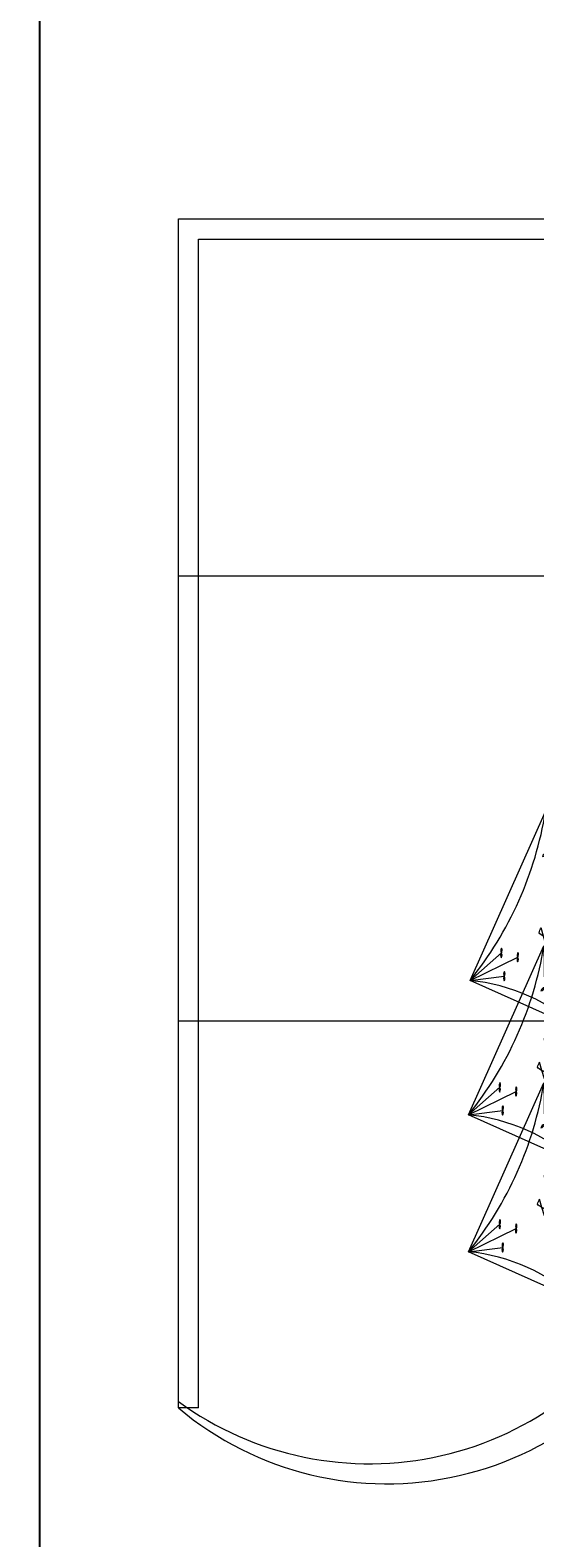
# Model space of a CAD drawing. Units: inches. Extents: x -61 to 1599, y -1316 to 257.
# Tile 54 of 204: x 215 to 240, y -408 to -334. Entities that reach past the tile are written whole.
import ezdxf

# ---------------------------------------------------------------- set-up
doc = ezdxf.new("R2010")
doc.units = ezdxf.units.IN
doc.header["$MEASUREMENT"] = 0
doc.layers.add('A-ANNO-DIMS', color=2, linetype='Continuous', lineweight=18)
doc.layers.add('FURNITURE', color=83, linetype='Continuous', lineweight=18)
doc.styles.get("Standard").update_dxf_attribs({"font": 'arial.ttf'})
doc.dimstyles.get("Standard").update_dxf_attribs({"dimtxt": 0.18, "dimasz": 0.18, "dimexe": 0.18, "dimexo": 0.0625, "dimgap": 0.09, "dimtad": 0, "dimtih": 1, "dimtoh": 1, "dimdec": 0, "dimzin": 0, "dimdsep": 46, "dimlunit": 3, "dimtxsty": 'Standard', "dimcen": 0.09, "dimadec": 0, "dimazin": 0, "dimtfac": 1, "dimtdec": 0, "dimtofl": 0, "dimtmove": 0, "dimatfit": 3, "dimfxl": 1, "dimtolj": 1, "dimtzin": 0, "dimarcsym": 0})

# ---------------------------------------------------------------- blocks, each defined once
blk = doc.blocks.new('MASTER-BEDROOM-CONSOLE')
for p, q in [((0, 44.886), (23.587, 44.886)), ((23.587, 37.779), (23.587, 9.438)), ((23.587, 37.779), (24.943, 35.589)), ((24.943, 35.589), (24.943, 9.456)), ((18.162, 33.228), (18.879, 30.704)), ((18.162, 33.228), (19.133, 31.826)), ((18.162, 33.228), (18.181, 31.167)), ((23.587, 30.804), (21.228, 29.654)), ((23.587, 30.804), (21.894, 30.592)), ((23.587, 30.804), (22.038, 29.443)), ((18.441, 28.869), (18.678, 29.228)), ((18.203, 28.51), (18.441, 28.869)), ((19.963, 28.553), (19.841, 28.966)), ((20.085, 28.141), (19.963, 28.553)), ((19.008, 27.84), (18.615, 28.016)), ((19.008, 27.84), (18.707, 27.533)), ((19.008, 27.84), (18.833, 27.448)), ((19.008, 27.84), (18.886, 28.253)), ((19.184, 28.233), (19.008, 27.84)), ((19.309, 28.148), (19.008, 27.84)), ((19.401, 27.665), (19.008, 27.84)), ((19.13, 27.428), (19.008, 27.84)), ((18.061, 27.072), (17.939, 27.485)), ((18.183, 26.66), (18.061, 27.072)), ((19.38, 26.517), (19.618, 26.876)), ((19.618, 26.876), (19.855, 27.235)), ((14.429, 24.877), (15.978, 26.238)), ((18.084, 26.588), (18.801, 24.064)), ((18.084, 26.588), (19.055, 25.186)), ((18.084, 26.588), (18.103, 24.527)), ((14.429, 24.877), (16.788, 26.026)), ((14.429, 24.877), (16.122, 25.089)), ((19.854, 22.452), (19.137, 24.976)), ((19.854, 22.452), (18.883, 23.854)), ((19.854, 22.452), (19.835, 24.514)), ((23.509, 24.163), (21.15, 23.014)), ((23.509, 24.163), (21.816, 23.952)), ((23.509, 24.163), (21.96, 22.803)), ((0, 22.886), (23.587, 22.886)), ((18.362, 22.229), (18.6, 22.588)), ((18.125, 21.87), (18.362, 22.229)), ((18.93, 21.2), (18.808, 21.613)), ((19.885, 21.913), (19.763, 22.326)), ((20.007, 21.5), (19.885, 21.913)), ((18.93, 21.2), (18.537, 21.376)), ((18.93, 21.2), (18.629, 20.893)), ((18.93, 21.2), (18.754, 20.808)), ((19.105, 21.593), (18.93, 21.2)), ((19.23, 21.508), (18.93, 21.2)), ((19.322, 21.025), (18.93, 21.2)), ((19.052, 20.788), (18.93, 21.2)), ((17.983, 20.432), (17.861, 20.845)), ((18.105, 20.02), (17.983, 20.432)), ((19.302, 19.877), (19.54, 20.236)), ((19.54, 20.236), (19.777, 20.595)), ((14.351, 18.237), (15.9, 19.598)), ((14.351, 18.237), (16.71, 19.386)), ((18.084, 19.819), (18.801, 17.295)), ((18.084, 19.819), (19.055, 18.417)), ((18.084, 19.819), (18.103, 17.757)), ((14.351, 18.237), (16.043, 18.448)), ((19.776, 15.812), (19.059, 18.336)), ((19.776, 15.812), (18.804, 17.214)), ((19.776, 15.812), (19.757, 17.874)), ((23.509, 17.394), (21.15, 16.245)), ((23.509, 17.394), (21.816, 17.183)), ((23.509, 17.394), (21.96, 16.033)), ((18.362, 15.459), (18.6, 15.818)), ((18.125, 15.101), (18.362, 15.459)), ((19.885, 15.143), (19.763, 15.556)), ((20.007, 14.731), (19.885, 15.143)), ((18.93, 14.431), (18.537, 14.606)), ((18.93, 14.431), (18.629, 14.123)), ((18.93, 14.431), (18.754, 14.038)), ((18.93, 14.431), (18.808, 14.843)), ((19.105, 14.823), (18.93, 14.431)), ((19.23, 14.738), (18.93, 14.431)), ((19.322, 14.255), (18.93, 14.431)), ((19.052, 14.018), (18.93, 14.431)), ((17.983, 13.663), (17.861, 14.075)), ((18.105, 13.25), (17.983, 13.663)), ((19.302, 13.108), (19.54, 13.466)), ((19.54, 13.466), (19.777, 13.825)), ((14.351, 11.468), (15.9, 12.828)), ((14.351, 11.468), (16.71, 12.617)), ((14.351, 11.468), (16.043, 11.679)), ((19.776, 9.043), (19.059, 11.567)), ((19.776, 9.043), (18.804, 10.445)), ((19.776, 9.043), (19.757, 11.104)), ((22.587, 9.438), (23.587, 9.438)), ((1, 3.748), (0, 3.748))]:
    blk.add_line(p, q)
for points in [[(0, 3.748), (0, 62.524), (23.587, 62.524), (23.587, 9.438)], [(1, 3.748), (1, 61.524), (22.587, 61.524), (22.587, 9.438)]]:
    blk.add_lwpolyline(points)
for points in [[(14.429, 24.877), (18.162, 33.228), (23.587, 30.804), (19.854, 22.452)], [(14.351, 18.237), (18.084, 26.588), (23.509, 24.163), (19.776, 15.812)], [(14.351, 11.468), (18.084, 19.819), (23.509, 17.394), (19.776, 9.043)]]:
    blk.add_lwpolyline(points, close=True)
for centre, radius in [((19.008, 27.84), 0.567), ((19.008, 27.84), 0.567), ((19.008, 27.84), 0.43), ((18.93, 21.2), 0.567), ((18.93, 21.2), 0.567), ((18.93, 21.2), 0.43), ((18.93, 14.431), 0.567), ((18.93, 14.431), 0.567), ((18.93, 14.431), 0.43)]:
    blk.add_circle(centre, radius)
for centre, radius, start, end in [((0.46, 36.131), 17.938, 321.14464, 350.6879), ((24.495, 40.115), 9.356, 227.40134, 264.43121), ((18.143, 31.378), 0.214, 280.21251, 346.40619), ((18.385, 31.121), 0.209, 99.3213, 167.2974), ((19.167, 31.62), 0.209, 99.3213, 167.2974), ((18.925, 31.877), 0.214, 280.21251, 346.40619), ((19.095, 32.037), 0.214, 280.21251, 346.40619), ((19.338, 31.78), 0.209, 99.3213, 167.2974), ((18.215, 30.96), 0.209, 99.3213, 167.2974), ((17.973, 31.217), 0.214, 280.21251, 346.40619), ((18.913, 30.498), 0.209, 99.3213, 167.2974), ((18.67, 30.755), 0.214, 280.21251, 346.40619), ((18.841, 30.915), 0.214, 280.21251, 346.40619), ((19.083, 30.658), 0.209, 99.3213, 167.2974), ((37.556, 19.55), 17.938, 141.14464, 170.6879), ((22.071, 30.471), 0.214, 145.42636, 211.62004), ((22.077, 30.705), 0.214, 145.42636, 211.62004), ((21.718, 30.48), 0.209, 324.53515, 32.51125), ((21.724, 30.714), 0.209, 324.53515, 32.51125), ((21.411, 29.767), 0.214, 145.42636, 211.62004), ((21.058, 29.776), 0.209, 324.53515, 32.51125), ((21.405, 29.533), 0.214, 145.42636, 211.62004), ((21.052, 29.542), 0.209, 324.53515, 32.51125), ((22.215, 29.321), 0.214, 145.42636, 211.62004), ((22.221, 29.555), 0.214, 145.42636, 211.62004), ((21.861, 29.33), 0.209, 324.53515, 32.51125), ((21.867, 29.564), 0.209, 324.53515, 32.51125), ((0.382, 29.491), 17.938, 321.14464, 350.6879), ((16.149, 26.117), 0.209, 144.53515, 212.51125), ((16.155, 26.351), 0.209, 144.53515, 212.51125), ((15.796, 26.126), 0.214, 325.42636, 31.62004), ((15.802, 26.36), 0.214, 325.42636, 31.62004), ((16.965, 26.139), 0.209, 144.53515, 212.51125), ((16.611, 26.148), 0.214, 325.42636, 31.62004), ((24.416, 33.475), 9.356, 227.40134, 264.43121), ((16.959, 25.905), 0.209, 144.53515, 212.51125), ((16.605, 25.914), 0.214, 325.42636, 31.62004), ((19.017, 25.397), 0.214, 280.21251, 346.40619), ((19.259, 25.14), 0.209, 99.3213, 167.2974), ((13.521, 15.565), 9.356, 47.40134, 84.43121), ((16.292, 24.967), 0.209, 144.53515, 212.51125), ((16.298, 25.201), 0.209, 144.53515, 212.51125), ((15.939, 24.976), 0.214, 325.42636, 31.62004), ((15.945, 25.21), 0.214, 325.42636, 31.62004), ((18.065, 24.738), 0.214, 280.21251, 346.40619), ((18.307, 24.48), 0.209, 99.3213, 167.2974), ((19.089, 24.98), 0.209, 99.3213, 167.2974), ((18.847, 25.237), 0.214, 280.21251, 346.40619), ((19.175, 24.765), 0.214, 100.21251, 166.40619), ((18.933, 25.022), 0.209, 279.3213, 347.2974), ((19.103, 25.183), 0.209, 279.3213, 347.2974), ((19.346, 24.926), 0.214, 100.21251, 166.40619), ((19.801, 24.721), 0.209, 279.3213, 347.2974), ((20.043, 24.464), 0.214, 100.21251, 166.40619), ((18.137, 24.32), 0.209, 99.3213, 167.2974), ((17.894, 24.577), 0.214, 280.21251, 346.40619), ((18.834, 23.858), 0.209, 99.3213, 167.2974), ((18.592, 24.115), 0.214, 280.21251, 346.40619), ((18.921, 23.643), 0.214, 100.21251, 166.40619), ((18.678, 23.9), 0.209, 279.3213, 347.2974), ((18.763, 24.275), 0.214, 280.21251, 346.40619), ((19.005, 24.018), 0.209, 99.3213, 167.2974), ((18.849, 24.061), 0.209, 279.3213, 347.2974), ((19.091, 23.804), 0.214, 100.21251, 166.40619), ((19.873, 24.303), 0.214, 100.21251, 166.40619), ((19.631, 24.56), 0.209, 279.3213, 347.2974), ((37.478, 12.91), 17.938, 141.14464, 170.6879), ((21.993, 23.83), 0.214, 145.42636, 211.62004), ((21.999, 24.065), 0.214, 145.42636, 211.62004), ((21.64, 23.84), 0.209, 324.53515, 32.51125), ((21.646, 24.074), 0.209, 324.53515, 32.51125), ((21.332, 23.127), 0.214, 145.42636, 211.62004), ((20.979, 23.136), 0.209, 324.53515, 32.51125), ((21.326, 22.892), 0.214, 145.42636, 211.62004), ((20.973, 22.902), 0.209, 324.53515, 32.51125), ((22.136, 22.681), 0.214, 145.42636, 211.62004), ((22.142, 22.915), 0.214, 145.42636, 211.62004), ((21.783, 22.69), 0.209, 324.53515, 32.51125), ((21.789, 22.924), 0.209, 324.53515, 32.51125), ((0.382, 22.721), 17.938, 321.14464, 350.6879), ((16.07, 19.476), 0.209, 144.53515, 212.51125), ((16.076, 19.711), 0.209, 144.53515, 212.51125), ((15.717, 19.486), 0.214, 325.42636, 31.62004), ((15.723, 19.72), 0.214, 325.42636, 31.62004), ((16.88, 19.265), 0.209, 144.53515, 212.51125), ((16.886, 19.499), 0.209, 144.53515, 212.51125), ((16.527, 19.274), 0.214, 325.42636, 31.62004), ((16.533, 19.508), 0.214, 325.42636, 31.62004), ((24.416, 26.706), 9.356, 227.40134, 264.43121), ((16.22, 18.561), 0.209, 144.53515, 212.51125), ((15.867, 18.57), 0.214, 325.42636, 31.62004), ((13.443, 8.925), 9.356, 47.40134, 84.43121), ((16.214, 18.327), 0.209, 144.53515, 212.51125), ((15.861, 18.336), 0.214, 325.42636, 31.62004), ((18.065, 17.968), 0.214, 280.21251, 346.40619), ((18.307, 17.711), 0.209, 99.3213, 167.2974), ((19.089, 18.21), 0.209, 99.3213, 167.2974), ((18.847, 18.467), 0.214, 280.21251, 346.40619), ((19.097, 18.125), 0.214, 100.21251, 166.40619), ((18.855, 18.382), 0.209, 279.3213, 347.2974), ((19.017, 18.628), 0.214, 280.21251, 346.40619), ((19.259, 18.371), 0.209, 99.3213, 167.2974), ((19.025, 18.543), 0.209, 279.3213, 347.2974), ((19.267, 18.286), 0.214, 100.21251, 166.40619), ((19.723, 18.081), 0.209, 279.3213, 347.2974), ((19.965, 17.824), 0.214, 100.21251, 166.40619), ((18.137, 17.55), 0.209, 99.3213, 167.2974), ((17.894, 17.807), 0.214, 280.21251, 346.40619), ((18.834, 17.088), 0.209, 99.3213, 167.2974), ((18.592, 17.345), 0.214, 280.21251, 346.40619), ((18.842, 17.003), 0.214, 100.21251, 166.40619), ((18.6, 17.26), 0.209, 279.3213, 347.2974), ((18.763, 17.506), 0.214, 280.21251, 346.40619), ((19.005, 17.249), 0.209, 99.3213, 167.2974), ((18.771, 17.421), 0.209, 279.3213, 347.2974), ((19.013, 17.164), 0.214, 100.21251, 166.40619), ((19.795, 17.663), 0.214, 100.21251, 166.40619), ((19.552, 17.92), 0.209, 279.3213, 347.2974), ((37.478, 6.14), 17.938, 141.14464, 170.6879), ((21.993, 17.061), 0.214, 145.42636, 211.62004), ((21.999, 17.295), 0.214, 145.42636, 211.62004), ((21.64, 17.07), 0.209, 324.53515, 32.51125), ((21.646, 17.304), 0.209, 324.53515, 32.51125), ((21.332, 16.357), 0.214, 145.42636, 211.62004), ((20.979, 16.366), 0.209, 324.53515, 32.51125), ((21.326, 16.123), 0.214, 145.42636, 211.62004), ((20.973, 16.132), 0.209, 324.53515, 32.51125), ((22.136, 15.911), 0.214, 145.42636, 211.62004), ((22.142, 16.145), 0.214, 145.42636, 211.62004), ((21.783, 15.92), 0.209, 324.53515, 32.51125), ((21.789, 16.155), 0.209, 324.53515, 32.51125), ((16.07, 12.707), 0.209, 144.53515, 212.51125), ((16.076, 12.941), 0.209, 144.53515, 212.51125), ((15.717, 12.716), 0.214, 325.42636, 31.62004), ((15.723, 12.95), 0.214, 325.42636, 31.62004), ((16.886, 12.729), 0.209, 144.53515, 212.51125), ((16.533, 12.739), 0.214, 325.42636, 31.62004), ((16.88, 12.495), 0.209, 144.53515, 212.51125), ((16.527, 12.504), 0.214, 325.42636, 31.62004), ((13.443, 2.156), 9.356, 47.40134, 84.43121), ((16.214, 11.557), 0.209, 144.53515, 212.51125), ((16.22, 11.791), 0.209, 144.53515, 212.51125), ((15.861, 11.566), 0.214, 325.42636, 31.62004), ((15.867, 11.801), 0.214, 325.42636, 31.62004), ((19.097, 11.356), 0.214, 100.21251, 166.40619), ((18.855, 11.613), 0.209, 279.3213, 347.2974), ((19.025, 11.773), 0.209, 279.3213, 347.2974), ((19.267, 11.516), 0.214, 100.21251, 166.40619), ((19.723, 11.311), 0.209, 279.3213, 347.2974), ((19.965, 11.054), 0.214, 100.21251, 166.40619), ((18.842, 10.234), 0.214, 100.21251, 166.40619), ((18.6, 10.491), 0.209, 279.3213, 347.2974), ((18.771, 10.651), 0.209, 279.3213, 347.2974), ((19.013, 10.394), 0.214, 100.21251, 166.40619), ((19.795, 10.893), 0.214, 100.21251, 166.40619), ((19.552, 11.151), 0.209, 279.3213, 347.2974), ((10.308, 16.053), 16.053, 230.04489, 335.73444), ((9.449, 17.042), 16.053, 233.93821, 331.72641)]:
    blk.add_arc(centre, radius, start, end)
for points in [[(18.203, 28.51), (18.191, 28.604), (18.167, 28.791), (18.438, 28.884), (18.778, 28.897), (18.67, 29.157), (18.678, 29.228)], [(20.085, 28.141), (20.124, 28.226), (20.202, 28.398), (19.97, 28.566), (19.649, 28.679), (19.829, 28.896), (19.841, 28.966)], [(19.401, 27.665), (19.361, 27.75), (19.281, 27.921), (19.003, 27.854), (18.708, 27.683), (18.66, 27.961), (18.615, 28.016)], [(19.309, 28.148), (19.303, 28.054), (19.292, 27.866), (19.008, 27.825), (18.671, 27.876), (18.729, 27.6), (18.707, 27.533)], [(19.13, 27.428), (19.169, 27.514), (19.247, 27.685), (19.015, 27.854), (18.694, 27.966), (18.873, 28.183), (18.886, 28.253)], [(19.184, 28.233), (19.098, 28.193), (18.927, 28.113), (18.994, 27.835), (19.165, 27.54), (18.888, 27.492), (18.833, 27.448)], [(18.183, 26.66), (18.222, 26.746), (18.3, 26.917), (18.069, 27.086), (17.747, 27.198), (17.927, 27.415), (17.939, 27.485)], [(19.38, 26.517), (19.368, 26.611), (19.344, 26.798), (19.615, 26.891), (19.955, 26.904), (19.847, 27.164), (19.855, 27.235)], [(18.125, 21.87), (18.113, 21.964), (18.089, 22.151), (18.359, 22.244), (18.7, 22.257), (18.592, 22.517), (18.6, 22.588)], [(19.052, 20.788), (19.091, 20.874), (19.169, 21.045), (18.937, 21.214), (18.615, 21.326), (18.795, 21.543), (18.808, 21.613)], [(20.007, 21.5), (20.046, 21.586), (20.124, 21.758), (19.892, 21.926), (19.571, 22.039), (19.75, 22.256), (19.763, 22.326)], [(19.322, 21.025), (19.283, 21.11), (19.203, 21.281), (18.924, 21.214), (18.63, 21.043), (18.582, 21.321), (18.537, 21.376)], [(19.23, 21.508), (19.225, 21.414), (19.213, 21.226), (18.93, 21.185), (18.593, 21.236), (18.651, 20.96), (18.629, 20.893)], [(19.105, 21.593), (19.02, 21.553), (18.849, 21.473), (18.916, 21.195), (19.087, 20.9), (18.809, 20.852), (18.754, 20.808)], [(18.105, 20.02), (18.144, 20.105), (18.222, 20.277), (17.99, 20.445), (17.669, 20.558), (17.848, 20.775), (17.861, 20.845)], [(19.302, 19.877), (19.29, 19.971), (19.266, 20.158), (19.537, 20.251), (19.877, 20.264), (19.769, 20.524), (19.777, 20.595)], [(18.125, 15.101), (18.113, 15.194), (18.089, 15.381), (18.359, 15.474), (18.7, 15.488), (18.592, 15.748), (18.6, 15.818)], [(20.007, 14.731), (20.046, 14.817), (20.124, 14.988), (19.892, 15.157), (19.571, 15.269), (19.75, 15.486), (19.763, 15.556)], [(19.322, 14.255), (19.283, 14.341), (19.203, 14.511), (18.924, 14.445), (18.63, 14.274), (18.582, 14.551), (18.537, 14.606)], [(19.23, 14.738), (19.225, 14.644), (19.213, 14.456), (18.93, 14.416), (18.593, 14.466), (18.651, 14.191), (18.629, 14.123)], [(19.052, 14.018), (19.091, 14.104), (19.169, 14.276), (18.937, 14.444), (18.615, 14.557), (18.795, 14.773), (18.808, 14.843)], [(19.105, 14.823), (19.02, 14.784), (18.849, 14.704), (18.916, 14.425), (19.087, 14.131), (18.809, 14.083), (18.754, 14.038)], [(18.105, 13.25), (18.144, 13.336), (18.222, 13.508), (17.99, 13.676), (17.669, 13.788), (17.848, 14.005), (17.861, 14.075)], [(19.302, 13.108), (19.29, 13.201), (19.266, 13.388), (19.537, 13.481), (19.877, 13.495), (19.769, 13.755), (19.777, 13.825)]]:
    blk.add_open_spline(points, degree=3, knots=[0, 0, 0, 0, 0.249187, 0.498374, 0.766554, 1.034734, 1.034734, 1.034734, 1.034734])
blk = doc.blocks.new('*D687')
at = {"layer": 'A-ANNO-DIMS', "color": 0, "lineweight": -2, "transparency": 16777216}
for p, q in [((289.418, 181.677), (-61.077, 181.677)), ((-60.897, 181.497), (-60.897, -528.952)), ((-60.897, -1239.765), (-60.897, -529.316)), ((319.64, -1239.945), (-61.077, -1239.945))]:
    blk.add_line(p, q, dxfattribs=at)
at = {"layer": 'A-ANNO-DIMS', "color": 0, "transparency": 16777216}
for points in [[(-60.927, 181.497), (-60.867, 181.497), (-60.897, 181.677)], [(-60.927, -1239.765), (-60.867, -1239.765), (-60.897, -1239.945)]]:
    blk.add_solid(points, dxfattribs=at)
at = {"layer": 'DEFPOINTS', "color": 0, "transparency": 16777216}
for p in [(289.481, 181.677), (-60.897, -1239.945), (319.703, -1239.945)]:
    blk.add_point(p, dxfattribs=at)
at = {"layer": 'A-ANNO-DIMS', "color": 0, "transparency": 16777216, "insert": (-60.897, -529.134), "char_height": 0.18, "attachment_point": 5}
blk.add_mtext('\\A1;1421.6', dxfattribs=at)
blk = doc.blocks.new('*D699')
at = {"layer": 'A-ANNO-DIMS', "color": 0, "lineweight": -2, "transparency": 16777216}
for p, q in [((835.64, -167.169), (-61.077, -167.169)), ((-60.897, -167.349), (-60.897, -306.726)), ((-60.897, -446.466), (-60.897, -307.09)), ((841.64, -446.646), (-61.077, -446.646))]:
    blk.add_line(p, q, dxfattribs=at)
at = {"layer": 'A-ANNO-DIMS', "color": 0, "transparency": 16777216}
for points in [[(-60.927, -167.349), (-60.867, -167.349), (-60.897, -167.169)], [(-60.927, -446.466), (-60.867, -446.466), (-60.897, -446.646)]]:
    blk.add_solid(points, dxfattribs=at)
at = {"layer": 'DEFPOINTS', "color": 0, "transparency": 16777216}
for p in [(835.703, -167.169), (-60.897, -446.646), (841.703, -446.646)]:
    blk.add_point(p, dxfattribs=at)
at = {"layer": 'A-ANNO-DIMS', "color": 0, "transparency": 16777216, "insert": (-60.897, -306.908), "char_height": 0.18, "attachment_point": 5}
blk.add_mtext('\\A1;279.5', dxfattribs=at)
blk = doc.blocks.new('*D701')
at = {"layer": 'A-ANNO-DIMS', "color": 0, "lineweight": -2, "transparency": 16777216}
for p, q in [((215.752, -616.882), (215.752, 257.457)), ((215.932, 257.277), (233.924, 257.277)), ((252.702, 257.277), (234.711, 257.277)), ((252.882, -616.882), (252.882, 257.457))]:
    blk.add_line(p, q, dxfattribs=at)
at = {"layer": 'A-ANNO-DIMS', "color": 0, "transparency": 16777216}
for points in [[(215.932, 257.307), (215.932, 257.247), (215.752, 257.277)], [(252.702, 257.307), (252.702, 257.247), (252.882, 257.277)]]:
    blk.add_solid(points, dxfattribs=at)
at = {"layer": 'DEFPOINTS', "color": 0, "transparency": 16777216}
for p in [(252.882, 257.277), (215.752, -616.945), (252.882, -616.945)]:
    blk.add_point(p, dxfattribs=at)
at = {"layer": 'A-ANNO-DIMS', "color": 0, "transparency": 16777216, "insert": (234.317, 257.277), "char_height": 0.18, "attachment_point": 5}
blk.add_mtext('\\A1;37.13', dxfattribs=at)

msp = doc.modelspace()

# ---------------------------------------------------------------- block references
at = {"layer": 'FURNITURE'}
msp.add_blockref('MASTER-BEDROOM-CONSOLE', (222.602, -405.667), dxfattribs=at)

# ---------------------------------------------------------------- dimensions: what is measured, and where the dimension line sits
at = {"layer": 'A-ANNO-DIMS'}
dim = msp.add_linear_dim(base=(252.8825, 257.2771), p1=(215.7521, -616.9446), p2=(252.8825, -616.9446), dimstyle='Standard', override={"dimdec": 2, "dimlfac": 1, "dimrnd": 0, "dimzin": 0, "dimdsep": 46, "dimlunit": 2}, dxfattribs=at)
dim.commit()
dim.dimension.update_dxf_attribs({"geometry": '*D701', "text_midpoint": (234.3173, 257.2771)})
for base, p1, p2, picture, middle in [((-60.8972, -1239.9446), (289.4807, 181.6771), (319.7028, -1239.9446), '*D687', (-60.8972, -529.1337)), ((-60.8972, -446.6462), (835.7028, -167.169), (841.7028, -446.6462), '*D699', (-60.8972, -306.9076))]:
    dim = msp.add_linear_dim(base=base, p1=p1, p2=p2, angle=90, dimstyle='Standard', override={"dimdec": 1, "dimlfac": 1, "dimrnd": 0, "dimzin": 0, "dimdsep": 46, "dimlunit": 2}, dxfattribs=at)
    dim.commit()
    dim.dimension.update_dxf_attribs({"geometry": picture, "text_midpoint": middle})

doc.saveas('drawing.dxf')
